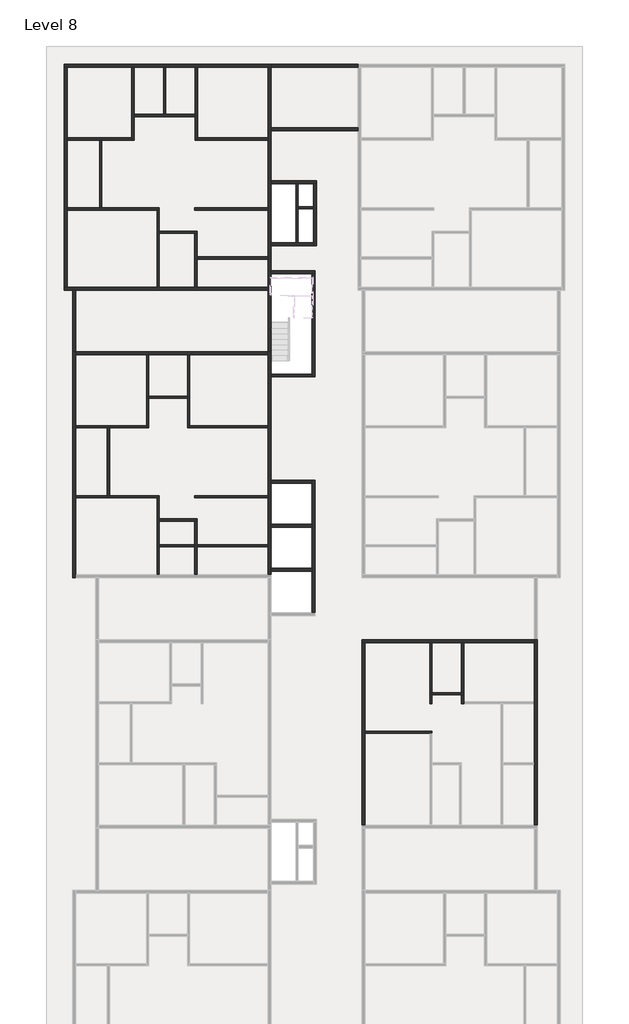
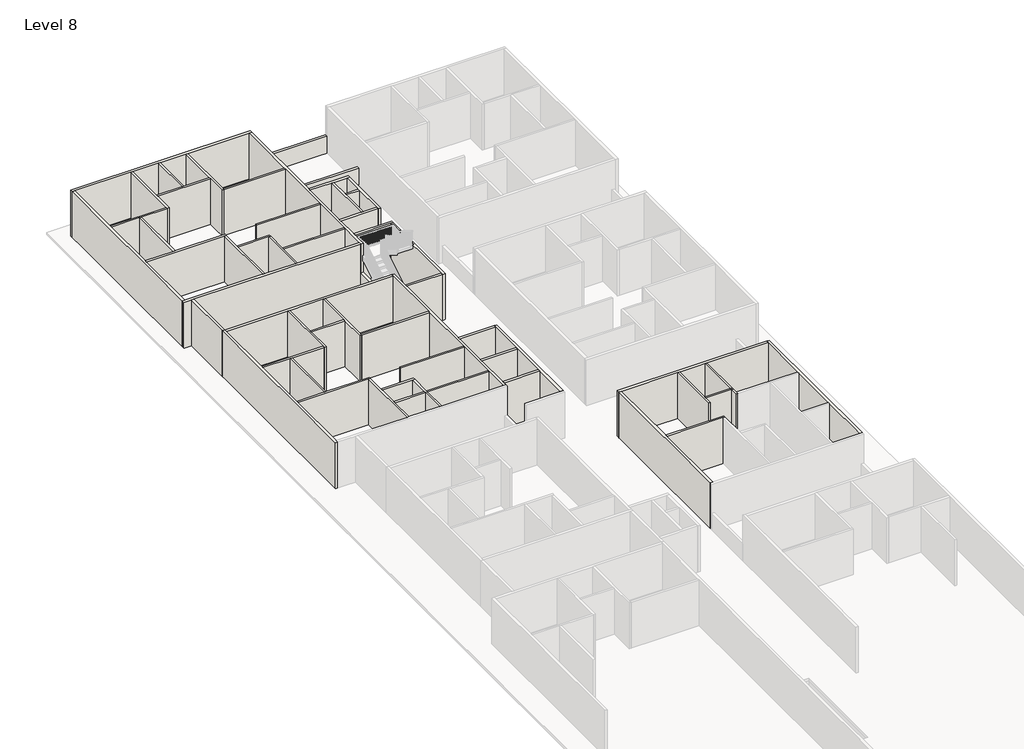
# One storey, part 3 of 8: 57 walls.
"""IFC4 building model written with IfcOpenShell, lengths in millimetres."""

from ifc_helpers import new_model, si_unit, frame, origin, place, context, project, spatial, polyline, outline, extrude, faceted_brep, element, save

model = new_model("IFC4")

# Units and contexts
model_context = context("Model", 3, world=origin())
ifc_project = project(units=[si_unit("LENGTHUNIT", "METRE", prefix="MILLI")], contexts=[model_context])

# Site, building, storey
site = spatial("IfcSite", under=ifc_project)
building = spatial("IfcBuilding", under=site)
storey = spatial("IfcBuildingStorey", under=building, Name="Level 8", Elevation=46570.6172466)

# Walls
placement = place(None, origin())
element("IfcWall", 1, ObjectType="4.5\"", at=placement, inside=storey, context=model_context, shape_type="Brep", body=[
    faceted_brep([(-10818.3415084, 35031.1216096, 46570.6172466), (-10818.3415084, 31373.5216096, 46570.6172466), (-10818.3415084, 31259.2216096, 46570.6172466), (-10818.3415084, 31259.2216096, 49618.6172466), (-10818.3415084, 31373.5216096, 49618.6172466), (-10818.3415084, 35031.1216096, 49618.6172466), (-10704.0415084, 35031.1216096, 46570.6172466), (-10704.0415084, 35031.1216096, 49618.6172466), (-10704.0415084, 32592.7216096, 49618.6172466), (-10704.0415084, 32478.4216096, 49618.6172466), (-10704.0415084, 31259.2216096, 49618.6172466), (-10704.0415084, 31259.2216096, 46570.6172466), (-10704.0415084, 32478.4216096, 46570.6172466), (-10704.0415084, 32592.7216096, 46570.6172466)], [[[0, 1, 2, 3, 4, 5]], [[6, 7, 8, 9, 10, 11, 12, 13]], [[2, 1, 0, 6, 13, 12, 11]], [[0, 5, 7, 6]], [[3, 2, 11, 10]], [[5, 4, 3, 10, 9, 8, 7]]]),
])
element("IfcWall", 2, ObjectType="4.5\"", at=placement, inside=storey, context=model_context, shape_type="Brep", body=[
    faceted_brep([(-10818.3415084, 31373.5216096, 46570.6172466), (-14171.1415084, 31373.5216096, 46570.6172466), (-14171.1415084, 31373.5216096, 49618.6172466), (-10818.3415084, 31373.5216096, 49618.6172466), (-10818.3415084, 31259.2216096, 46570.6172466), (-10818.3415084, 31259.2216096, 49618.6172466), (-12380.4415084, 31259.2216096, 49618.6172466), (-12494.7415084, 31259.2216096, 49618.6172466), (-14171.1415084, 31259.2216096, 49618.6172466), (-14171.1415084, 31259.2216096, 46570.6172466), (-12494.7415084, 31259.2216096, 46570.6172466), (-12380.4415084, 31259.2216096, 46570.6172466)], [[[0, 1, 2, 3]], [[4, 5, 6, 7, 8, 9, 10, 11]], [[1, 0, 4, 11, 10, 9]], [[0, 3, 5, 4]], [[2, 1, 9, 8]], [[3, 2, 8, 7, 6, 5]]]),
])
element("IfcWall", 3, ObjectType="4.5\"", at=placement, inside=storey, context=model_context, shape_type="SweptSolid", body=[
    extrude(outline(polyline([(-12494.7415084, 27754.0216096), (-12494.7415084, 31259.2216096), (-12380.4415084, 31259.2216096), (-12380.4415084, 27754.0216096), (-12494.7415084, 27754.0216096)])), frame((0.0, 0.0, 46570.6172466), z_axis=(0.0, 0.0, 1.0), x_axis=(1.0, 0.0, 0.0)), (0.0, 0.0, 1.0), 3048.0),
])
element("IfcWall", 4, ObjectType="4.5\"", at=placement, inside=storey, context=model_context, shape_type="Brep", body=[
    faceted_brep([(-14171.1415084, 27639.7216096, 46570.6172466), (-9510.2415084, 27639.7216096, 46570.6172466), (-9395.9415084, 27639.7216096, 46570.6172466), (-9395.9415084, 27639.7216096, 49618.6172466), (-9510.2415084, 27639.7216096, 49618.6172466), (-14171.1415084, 27639.7216096, 49618.6172466), (-14171.1415084, 27754.0216096, 46570.6172466), (-14171.1415084, 27754.0216096, 49618.6172466), (-12494.7415084, 27754.0216096, 49618.6172466), (-12380.4415084, 27754.0216096, 49618.6172466), (-9395.9415084, 27754.0216096, 49618.6172466), (-9395.9415084, 27754.0216096, 46570.6172466), (-12380.4415084, 27754.0216096, 46570.6172466), (-12494.7415084, 27754.0216096, 46570.6172466)], [[[0, 1, 2, 3, 4, 5]], [[6, 7, 8, 9, 10, 11, 12, 13]], [[2, 1, 0, 6, 13, 12, 11]], [[0, 5, 7, 6]], [[3, 2, 11, 10]], [[5, 4, 3, 10, 9, 8, 7]]]),
])
element("IfcWall", 5, ObjectType="4.5\"", at=placement, inside=storey, context=model_context, shape_type="Brep", body=[
    faceted_brep([(-9510.2415084, 27639.7216096, 46570.6172466), (-9510.2415084, 23651.9216096, 46570.6172466), (-9510.2415084, 23651.9216096, 49618.6172466), (-9510.2415084, 27639.7216096, 49618.6172466), (-9395.9415084, 27639.7216096, 46570.6172466), (-9395.9415084, 27639.7216096, 49618.6172466), (-9395.9415084, 26547.5216096, 49618.6172466), (-9395.9415084, 26433.2216096, 49618.6172466), (-9395.9415084, 23651.9216096, 49618.6172466), (-9395.9415084, 23651.9216096, 46570.6172466), (-9395.9415084, 26433.2216096, 46570.6172466), (-9395.9415084, 26547.5216096, 46570.6172466)], [[[0, 1, 2, 3]], [[4, 5, 6, 7, 8, 9, 10, 11]], [[1, 0, 4, 11, 10, 9]], [[0, 3, 5, 4]], [[2, 1, 9, 8]], [[3, 2, 8, 7, 6, 5]]]),
])
element("IfcWall", 6, ObjectType="4.5\"", at=placement, inside=storey, context=model_context, shape_type="Brep", body=[
    faceted_brep([(-9395.9415084, 26433.2216096, 46570.6172466), (-7567.1415084, 26433.2216096, 46570.6172466), (-7452.8415084, 26433.2216096, 46570.6172466), (-7452.8415084, 26433.2216096, 49618.6172466), (-7567.1415084, 26433.2216096, 49618.6172466), (-9395.9415084, 26433.2216096, 49618.6172466), (-9395.9415084, 26547.5216096, 46570.6172466), (-9395.9415084, 26547.5216096, 49618.6172466), (-7452.8415084, 26547.5216096, 49618.6172466), (-7452.8415084, 26547.5216096, 46570.6172466)], [[[0, 1, 2, 3, 4, 5]], [[6, 7, 8, 9]], [[2, 1, 0, 6, 9]], [[0, 5, 7, 6]], [[3, 2, 9, 8]], [[5, 4, 3, 8, 7]]]),
])
element("IfcWall", 7, ObjectType="4.5\"", at=placement, inside=storey, context=model_context, shape_type="Brep", body=[
    faceted_brep([(-7567.1415084, 26433.2216096, 46570.6172466), (-7567.1415084, 23651.9216096, 46570.6172466), (-7567.1415084, 23651.9216096, 49618.6172466), (-7567.1415084, 26433.2216096, 49618.6172466), (-7452.8415084, 26433.2216096, 46570.6172466), (-7452.8415084, 26433.2216096, 49618.6172466), (-7452.8415084, 25214.0216096, 49618.6172466), (-7452.8415084, 25099.7216096, 49618.6172466), (-7452.8415084, 23651.9216096, 49618.6172466), (-7452.8415084, 23651.9216096, 46570.6172466), (-7452.8415084, 25099.7216096, 46570.6172466), (-7452.8415084, 25214.0216096, 46570.6172466)], [[[0, 1, 2, 3]], [[4, 5, 6, 7, 8, 9, 10, 11]], [[1, 0, 4, 11, 10, 9]], [[0, 3, 5, 4]], [[2, 1, 9, 8]], [[3, 2, 8, 7, 6, 5]]]),
])
element("IfcWall", 8, ObjectType="4.5\"", at=placement, inside=storey, context=model_context, shape_type="SweptSolid", body=[
    extrude(outline(polyline([(-7452.8415084, 25214.0216096), (-3769.8415084, 25214.0216096), (-3769.8415084, 25099.7216096), (-7452.8415084, 25099.7216096), (-7452.8415084, 25214.0216096)])), frame((0.0, 0.0, 46570.6172466), z_axis=(0.0, 0.0, 1.0), x_axis=(1.0, 0.0, 0.0)), (0.0, 0.0, 1.0), 3048.0),
])
element("IfcWall", 9, ObjectType="4.5\"", at=placement, inside=storey, context=model_context, shape_type="SweptSolid", body=[
    extrude(outline(polyline([(-3769.8415084, 27639.7216096), (-7567.1415084, 27639.7216096), (-7567.1415084, 27754.0216096), (-3769.8415084, 27754.0216096), (-3769.8415084, 27639.7216096)])), frame((0.0, 0.0, 46570.6172466), z_axis=(0.0, 0.0, 1.0), x_axis=(1.0, 0.0, 0.0)), (0.0, 0.0, 1.0), 3048.0),
])
element("IfcWall", 10, ObjectType="4.5\"", at=placement, inside=storey, context=model_context, shape_type="Brep", body=[
    faceted_brep([(-10704.0415084, 32478.4216096, 46570.6172466), (-7541.7415084, 32478.4216096, 46570.6172466), (-7541.7415084, 32478.4216096, 49618.6172466), (-10704.0415084, 32478.4216096, 49618.6172466), (-10704.0415084, 32592.7216096, 46570.6172466), (-10704.0415084, 32592.7216096, 49618.6172466), (-9180.0415084, 32592.7216096, 49618.6172466), (-9065.7415084, 32592.7216096, 49618.6172466), (-7541.7415084, 32592.7216096, 49618.6172466), (-7541.7415084, 32592.7216096, 46570.6172466), (-9065.7415084, 32592.7216096, 46570.6172466), (-9180.0415084, 32592.7216096, 46570.6172466)], [[[0, 1, 2, 3]], [[4, 5, 6, 7, 8, 9, 10, 11]], [[1, 0, 4, 11, 10, 9]], [[0, 3, 5, 4]], [[2, 1, 9, 8]], [[3, 2, 8, 7, 6, 5]]]),
])
element("IfcWall", 11, ObjectType="4.5\"", at=placement, inside=storey, context=model_context, shape_type="SweptSolid", body=[
    extrude(outline(polyline([(-9180.0415084, 32592.7216096), (-9180.0415084, 35031.1216096), (-9065.7415084, 35031.1216096), (-9065.7415084, 32592.7216096), (-9180.0415084, 32592.7216096)])), frame((0.0, 0.0, 46570.6172466), z_axis=(0.0, 0.0, 1.0), x_axis=(1.0, 0.0, 0.0)), (0.0, 0.0, 1.0), 3048.0),
])
element("IfcWall", 12, ObjectType="4.5\"", at=placement, inside=storey, context=model_context, shape_type="Brep", body=[
    faceted_brep([(-7541.7415084, 35031.1216096, 46570.6172466), (-7541.7415084, 32592.7216096, 46570.6172466), (-7541.7415084, 32478.4216096, 46570.6172466), (-7541.7415084, 31259.2216096, 46570.6172466), (-7541.7415084, 31259.2216096, 49618.6172466), (-7541.7415084, 32478.4216096, 49618.6172466), (-7541.7415084, 32592.7216096, 49618.6172466), (-7541.7415084, 35031.1216096, 49618.6172466), (-7427.4415084, 35031.1216096, 46570.6172466), (-7427.4415084, 35031.1216096, 49618.6172466), (-7427.4415084, 31373.5216096, 49618.6172466), (-7427.4415084, 31259.2216096, 49618.6172466), (-7427.4415084, 31259.2216096, 46570.6172466), (-7427.4415084, 31373.5216096, 46570.6172466)], [[[0, 1, 2, 3, 4, 5, 6, 7]], [[8, 9, 10, 11, 12, 13]], [[3, 2, 1, 0, 8, 13, 12]], [[0, 7, 9, 8]], [[4, 3, 12, 11]], [[7, 6, 5, 4, 11, 10, 9]]]),
])
element("IfcWall", 13, ObjectType="4.5\"", at=placement, inside=storey, context=model_context, shape_type="SweptSolid", body=[
    extrude(outline(polyline([(-3769.8415084, 31259.2216096), (-7427.4415084, 31259.2216096), (-7427.4415084, 31373.5216096), (-3769.8415084, 31373.5216096), (-3769.8415084, 31259.2216096)])), frame((0.0, 0.0, 46570.6172466), z_axis=(0.0, 0.0, 1.0), x_axis=(1.0, 0.0, 0.0)), (0.0, 0.0, 1.0), 3048.0),
])
element("IfcWall", 14, ObjectType="4.5\"", at=placement, inside=storey, context=model_context, shape_type="Brep", body=[
    faceted_brep([(-10061.4044854, 20146.7216096, 46570.6172466), (-10061.4044854, 16489.1216096, 46570.6172466), (-10061.4044854, 16374.8216096, 46570.6172466), (-10061.4044854, 16374.8216096, 49618.6172466), (-10061.4044854, 16489.1216096, 49618.6172466), (-10061.4044854, 20146.7216096, 49618.6172466), (-9947.1044854, 20146.7216096, 46570.6172466), (-9947.1044854, 20146.7216096, 49618.6172466), (-9947.1044854, 18013.1216096, 49618.6172466), (-9947.1044854, 17898.8216096, 49618.6172466), (-9947.1044854, 16374.8216096, 49618.6172466), (-9947.1044854, 16374.8216096, 46570.6172466), (-9947.1044854, 17898.8216096, 46570.6172466), (-9947.1044854, 18013.1216096, 46570.6172466)], [[[0, 1, 2, 3, 4, 5]], [[6, 7, 8, 9, 10, 11, 12, 13]], [[2, 1, 0, 6, 13, 12, 11]], [[0, 5, 7, 6]], [[3, 2, 11, 10]], [[5, 4, 3, 10, 9, 8, 7]]]),
])
element("IfcWall", 15, ObjectType="4.5\"", at=placement, inside=storey, context=model_context, shape_type="Brep", body=[
    faceted_brep([(-10061.4044854, 16489.1216096, 46570.6172466), (-13719.0044854, 16489.1216096, 46570.6172466), (-13719.0044854, 16489.1216096, 49618.6172466), (-10061.4044854, 16489.1216096, 49618.6172466), (-10061.4044854, 16374.8216096, 46570.6172466), (-10061.4044854, 16374.8216096, 49618.6172466), (-11980.3915084, 16374.8216096, 49618.6172466), (-12094.6915084, 16374.8216096, 49618.6172466), (-13719.0044854, 16374.8216096, 49618.6172466), (-13719.0044854, 16374.8216096, 46570.6172466), (-12094.6915084, 16374.8216096, 46570.6172466), (-11980.3915084, 16374.8216096, 46570.6172466)], [[[0, 1, 2, 3]], [[4, 5, 6, 7, 8, 9, 10, 11]], [[1, 0, 4, 11, 10, 9]], [[0, 3, 5, 4]], [[2, 1, 9, 8]], [[3, 2, 8, 7, 6, 5]]]),
])
element("IfcWall", 16, ObjectType="4.5\"", at=placement, inside=storey, context=model_context, shape_type="SweptSolid", body=[
    extrude(outline(polyline([(-7940.5044854, 17898.8216096), (-9947.1044854, 17898.8216096), (-9947.1044854, 18013.1216096), (-7940.5044854, 18013.1216096), (-7940.5044854, 17898.8216096)])), frame((0.0, 0.0, 46570.6172466), z_axis=(0.0, 0.0, 1.0), x_axis=(1.0, 0.0, 0.0)), (0.0, 0.0, 1.0), 3048.0),
])
element("IfcWall", 17, ObjectType="4.5\"", at=placement, inside=storey, context=model_context, shape_type="Brep", body=[
    faceted_brep([(-7940.5044854, 20146.7216096, 46570.6172466), (-7940.5044854, 18013.1216096, 46570.6172466), (-7940.5044854, 17898.8216096, 46570.6172466), (-7940.5044854, 16374.8216096, 46570.6172466), (-7940.5044854, 16374.8216096, 49618.6172466), (-7940.5044854, 17898.8216096, 49618.6172466), (-7940.5044854, 18013.1216096, 49618.6172466), (-7940.5044854, 20146.7216096, 49618.6172466), (-7826.2044854, 20146.7216096, 46570.6172466), (-7826.2044854, 20146.7216096, 49618.6172466), (-7826.2044854, 16489.1216096, 49618.6172466), (-7826.2044854, 16374.8216096, 49618.6172466), (-7826.2044854, 16374.8216096, 46570.6172466), (-7826.2044854, 16489.1216096, 46570.6172466)], [[[0, 1, 2, 3, 4, 5, 6, 7]], [[8, 9, 10, 11, 12, 13]], [[3, 2, 1, 0, 8, 13, 12]], [[0, 7, 9, 8]], [[4, 3, 12, 11]], [[7, 6, 5, 4, 11, 10, 9]]]),
])
element("IfcWall", 18, ObjectType="4.5\"", at=placement, inside=storey, context=model_context, shape_type="SweptSolid", body=[
    extrude(outline(polyline([(-3769.8415084, 16374.8216096), (-7826.2044854, 16374.8216096), (-7826.2044854, 16489.1216096), (-3769.8415084, 16489.1216096), (-3769.8415084, 16374.8216096)])), frame((0.0, 0.0, 46570.6172466), z_axis=(0.0, 0.0, 1.0), x_axis=(1.0, 0.0, 0.0)), (0.0, 0.0, 1.0), 3048.0),
])
element("IfcWall", 19, ObjectType="4.5\"", at=placement, inside=storey, context=model_context, shape_type="SweptSolid", body=[
    extrude(outline(polyline([(-12094.6915084, 12869.6216096), (-12094.6915084, 16374.8216096), (-11980.3915084, 16374.8216096), (-11980.3915084, 12869.6216096), (-12094.6915084, 12869.6216096)])), frame((0.0, 0.0, 46570.6172466), z_axis=(0.0, 0.0, 1.0), x_axis=(1.0, 0.0, 0.0)), (0.0, 0.0, 1.0), 3048.0),
])
element("IfcWall", 20, ObjectType="4.5\"", at=placement, inside=storey, context=model_context, shape_type="Brep", body=[
    faceted_brep([(-13719.0044854, 12755.3216096, 46570.6172466), (-9510.2415084, 12755.3216096, 46570.6172466), (-9395.9415084, 12755.3216096, 46570.6172466), (-9395.9415084, 12755.3216096, 49618.6172466), (-9510.2415084, 12755.3216096, 49618.6172466), (-13719.0044854, 12755.3216096, 49618.6172466), (-13719.0044854, 12869.6216096, 46570.6172466), (-13719.0044854, 12869.6216096, 49618.6172466), (-12094.6915084, 12869.6216096, 49618.6172466), (-11980.3915084, 12869.6216096, 49618.6172466), (-9395.9415084, 12869.6216096, 49618.6172466), (-9395.9415084, 12869.6216096, 46570.6172466), (-11980.3915084, 12869.6216096, 46570.6172466), (-12094.6915084, 12869.6216096, 46570.6172466)], [[[0, 1, 2, 3, 4, 5]], [[6, 7, 8, 9, 10, 11, 12, 13]], [[2, 1, 0, 6, 13, 12, 11]], [[0, 5, 7, 6]], [[3, 2, 11, 10]], [[5, 4, 3, 10, 9, 8, 7]]]),
])
element("IfcWall", 21, ObjectType="4.5\"", at=placement, inside=storey, context=model_context, shape_type="Brep", body=[
    faceted_brep([(-9510.2415084, 12755.3216096, 46570.6172466), (-9510.2415084, 8767.5216096, 46570.6172466), (-9510.2415084, 8767.5216096, 49618.6172466), (-9510.2415084, 12755.3216096, 49618.6172466), (-9395.9415084, 12755.3216096, 46570.6172466), (-9395.9415084, 12755.3216096, 49618.6172466), (-9395.9415084, 11663.1216096, 49618.6172466), (-9395.9415084, 11548.8216096, 49618.6172466), (-9395.9415084, 10329.6216096, 49618.6172466), (-9395.9415084, 10215.3216096, 49618.6172466), (-9395.9415084, 8767.5216096, 49618.6172466), (-9395.9415084, 8767.5216096, 46570.6172466), (-9395.9415084, 10215.3216096, 46570.6172466), (-9395.9415084, 10329.6216096, 46570.6172466), (-9395.9415084, 11548.8216096, 46570.6172466), (-9395.9415084, 11663.1216096, 46570.6172466)], [[[0, 1, 2, 3]], [[4, 5, 6, 7, 8, 9, 10, 11, 12, 13, 14, 15]], [[1, 0, 4, 15, 14, 13, 12, 11]], [[0, 3, 5, 4]], [[2, 1, 11, 10]], [[3, 2, 10, 9, 8, 7, 6, 5]]]),
])
element("IfcWall", 22, ObjectType="4.5\"", at=placement, inside=storey, context=model_context, shape_type="SweptSolid", body=[
    extrude(outline(polyline([(-7567.1415084, 10215.3216096), (-9395.9415084, 10215.3216096), (-9395.9415084, 10329.6216096), (-7567.1415084, 10329.6216096), (-7567.1415084, 10215.3216096)])), frame((0.0, 0.0, 46570.6172466), z_axis=(0.0, 0.0, 1.0), x_axis=(1.0, 0.0, 0.0)), (0.0, 0.0, 1.0), 3048.0),
])
element("IfcWall", 23, ObjectType="4.5\"", at=placement, inside=storey, context=model_context, shape_type="Brep", body=[
    faceted_brep([(-9395.9415084, 11548.8216096, 46570.6172466), (-7567.1415084, 11548.8216096, 46570.6172466), (-7452.8415084, 11548.8216096, 46570.6172466), (-7452.8415084, 11548.8216096, 49618.6172466), (-7567.1415084, 11548.8216096, 49618.6172466), (-9395.9415084, 11548.8216096, 49618.6172466), (-9395.9415084, 11663.1216096, 46570.6172466), (-9395.9415084, 11663.1216096, 49618.6172466), (-7452.8415084, 11663.1216096, 49618.6172466), (-7452.8415084, 11663.1216096, 46570.6172466)], [[[0, 1, 2, 3, 4, 5]], [[6, 7, 8, 9]], [[2, 1, 0, 6, 9]], [[0, 5, 7, 6]], [[3, 2, 9, 8]], [[5, 4, 3, 8, 7]]]),
])
element("IfcWall", 24, ObjectType="4.5\"", at=placement, inside=storey, context=model_context, shape_type="Brep", body=[
    faceted_brep([(-7567.1415084, 11548.8216096, 46570.6172466), (-7567.1415084, 10329.6216096, 46570.6172466), (-7567.1415084, 10215.3216096, 46570.6172466), (-7567.1415084, 8767.5216096, 46570.6172466), (-7567.1415084, 8767.5216096, 49618.6172466), (-7567.1415084, 10215.3216096, 49618.6172466), (-7567.1415084, 10329.6216096, 49618.6172466), (-7567.1415084, 11548.8216096, 49618.6172466), (-7452.8415084, 11548.8216096, 46570.6172466), (-7452.8415084, 11548.8216096, 49618.6172466), (-7452.8415084, 10329.6216096, 49618.6172466), (-7452.8415084, 10215.3216096, 49618.6172466), (-7452.8415084, 8767.5216096, 49618.6172466), (-7452.8415084, 8767.5216096, 46570.6172466), (-7452.8415084, 10215.3216096, 46570.6172466), (-7452.8415084, 10329.6216096, 46570.6172466)], [[[0, 1, 2, 3, 4, 5, 6, 7]], [[8, 9, 10, 11, 12, 13, 14, 15]], [[3, 2, 1, 0, 8, 15, 14, 13]], [[0, 7, 9, 8]], [[4, 3, 13, 12]], [[7, 6, 5, 4, 12, 11, 10, 9]]]),
])
element("IfcWall", 25, ObjectType="4.5\"", at=placement, inside=storey, context=model_context, shape_type="SweptSolid", body=[
    extrude(outline(polyline([(-3769.8415084, 10215.3216096), (-7452.8415084, 10215.3216096), (-7452.8415084, 10329.6216096), (-3769.8415084, 10329.6216096), (-3769.8415084, 10215.3216096)])), frame((0.0, 0.0, 46570.6172466), z_axis=(0.0, 0.0, 1.0), x_axis=(1.0, 0.0, 0.0)), (0.0, 0.0, 1.0), 3048.0),
])
element("IfcWall", 26, ObjectType="4.5\"", at=placement, inside=storey, context=model_context, shape_type="SweptSolid", body=[
    extrude(outline(polyline([(-3769.8415084, 12755.3216096), (-7567.1415084, 12755.3216096), (-7567.1415084, 12869.6216096), (-3769.8415084, 12869.6216096), (-3769.8415084, 12755.3216096)])), frame((0.0, 0.0, 46570.6172466), z_axis=(0.0, 0.0, 1.0), x_axis=(1.0, 0.0, 0.0)), (0.0, 0.0, 1.0), 3048.0),
])
element("IfcWall", 27, ObjectType="4.5\"", at=placement, inside=storey, context=model_context, shape_type="Brep", body=[
    faceted_brep([(1259.3584916, 572.7745083, 46570.6172466), (4610.8714687, 572.7745083, 46570.6172466), (4725.1714687, 572.7745083, 46570.6172466), (4725.1714687, 572.7745083, 49618.6172466), (4610.8714687, 572.7745083, 49618.6172466), (1259.3584916, 572.7745083, 49618.6172466), (1259.3584916, 687.0745083, 46570.6172466), (1259.3584916, 687.0745083, 49618.6172466), (4725.1714687, 687.0745083, 49618.6172466), (4725.1714687, 687.0745083, 46570.6172466)], [[[0, 1, 2, 3, 4, 5]], [[6, 7, 8, 9]], [[2, 1, 0, 6, 9]], [[0, 5, 7, 6]], [[3, 2, 9, 8]], [[5, 4, 3, 8, 7]]]),
])
element("IfcWall", 28, ObjectType="4.5\"", at=placement, inside=storey, context=model_context, shape_type="Brep", body=[
    faceted_brep([(4610.8714687, 5262.3216096, 46570.6172466), (4610.8714687, 2100.0216096, 46570.6172466), (4610.8714687, 2100.0216096, 49618.6172466), (4610.8714687, 5262.3216096, 49618.6172466), (4725.1714687, 5262.3216096, 46570.6172466), (4725.1714687, 5262.3216096, 49618.6172466), (4725.1714687, 2671.5216096, 49618.6172466), (4725.1714687, 2557.2216096, 49618.6172466), (4725.1714687, 2100.0216096, 49618.6172466), (4725.1714687, 2100.0216096, 46570.6172466), (4725.1714687, 2557.2216096, 46570.6172466), (4725.1714687, 2671.5216096, 46570.6172466)], [[[0, 1, 2, 3]], [[4, 5, 6, 7, 8, 9, 10, 11]], [[1, 0, 4, 11, 10, 9]], [[2, 1, 9, 8]], [[0, 3, 5, 4]], [[3, 2, 8, 7, 6, 5]]]),
])
element("IfcWall", 29, ObjectType="4.5\"", at=placement, inside=storey, context=model_context, shape_type="Brep", body=[
    faceted_brep([(4725.1714687, 2557.2216096, 46570.6172466), (6249.1714687, 2557.2216096, 46570.6172466), (6363.4714687, 2557.2216096, 46570.6172466), (6363.4714687, 2557.2216096, 49618.6172466), (6249.1714687, 2557.2216096, 49618.6172466), (4725.1714687, 2557.2216096, 49618.6172466), (4725.1714687, 2671.5216096, 46570.6172466), (4725.1714687, 2671.5216096, 49618.6172466), (6249.1714687, 2671.5216096, 49618.6172466), (6363.4714687, 2671.5216096, 49618.6172466), (6363.4714687, 2671.5216096, 46570.6172466), (6249.1714687, 2671.5216096, 46570.6172466)], [[[0, 1, 2, 3, 4, 5]], [[6, 7, 8, 9, 10, 11]], [[2, 1, 0, 6, 11, 10]], [[0, 5, 7, 6]], [[3, 2, 10, 9]], [[5, 4, 3, 9, 8, 7]]]),
])
element("IfcWall", 30, ObjectType="4.5\"", at=placement, inside=storey, context=model_context, shape_type="SweptSolid", body=[
    extrude(outline(polyline([(6363.4714687, 5262.3216096), (6363.4714687, 2671.5216096), (6249.1714687, 2671.5216096), (6249.1714687, 5262.3216096), (6363.4714687, 5262.3216096)])), frame((0.0, 0.0, 46570.6172466), z_axis=(0.0, 0.0, 1.0), x_axis=(1.0, 0.0, 0.0)), (0.0, 0.0, 1.0), 3048.0),
])
element("IfcWall", 31, ObjectType="4.5\"", at=placement, inside=storey, context=model_context, shape_type="Brep", body=[
    faceted_brep([(6249.1714687, 2557.2216096, 46570.6172466), (6249.1714687, 2100.0216096, 46570.6172466), (6249.1714687, 2100.0216096, 49618.6172466), (6249.1714687, 2557.2216096, 49618.6172466), (6363.4714687, 2557.2216096, 46570.6172466), (6363.4714687, 2557.2216096, 49618.6172466), (6363.4714687, 2214.3216096, 49618.6172466), (6363.4714687, 2100.0216096, 49618.6172466), (6363.4714687, 2100.0216096, 46570.6172466), (6363.4714687, 2214.3216096, 46570.6172466)], [[[0, 1, 2, 3]], [[4, 5, 6, 7, 8, 9]], [[1, 0, 4, 9, 8]], [[0, 3, 5, 4]], [[2, 1, 8, 7]], [[3, 2, 7, 6, 5]]]),
])
element("IfcWall", 32, ObjectType="4.5\"", at=placement, inside=storey, context=model_context, shape_type="Brep", body=[
    faceted_brep([(-2321.9738684, 29000.0900967, 46570.6172466), (-2321.9738684, 25952.0900967, 46570.6172466), (-2321.9738684, 25952.0900967, 49618.6172466), (-2321.9738684, 29000.0900967, 49618.6172466), (-2207.6738684, 29000.0900967, 46570.6172466), (-2207.6738684, 29000.0900967, 49618.6172466), (-2207.6738684, 27820.8172885, 49618.6172466), (-2207.6738684, 27706.5172885, 49618.6172466), (-2207.6738684, 25952.0900967, 49618.6172466), (-2207.6738684, 25952.0900967, 46570.6172466), (-2207.6738684, 27706.5172885, 46570.6172466), (-2207.6738684, 27820.8172885, 46570.6172466)], [[[0, 1, 2, 3]], [[4, 5, 6, 7, 8, 9, 10, 11]], [[1, 0, 4, 11, 10, 9]], [[3, 2, 8, 7, 6, 5]], [[0, 3, 5, 4]], [[2, 1, 9, 8]]]),
])
element("IfcWall", 33, ObjectType="4.5\"", at=placement, inside=storey, context=model_context, shape_type="SweptSolid", body=[
    extrude(outline(polyline([(-2207.6738684, 27820.8172885), (-1407.6415084, 27820.8172885), (-1407.6415084, 27706.5172885), (-2207.6738684, 27706.5172885), (-2207.6738684, 27820.8172885)])), frame((0.0, 0.0, 46570.6172466), z_axis=(0.0, 0.0, 1.0), x_axis=(1.0, 0.0, 0.0)), (0.0, 0.0, 1.0), 3048.0),
])
element("IfcWall", 34, ObjectType="6\"", at=placement, inside=storey, context=model_context, shape_type="Brep", body=[
    faceted_brep([(-14323.5415084, 35031.1216096, 46570.6172466), (-14171.1415084, 35031.1216096, 46570.6172466), (-10818.3415084, 35031.1216096, 46570.6172466), (-10704.0415084, 35031.1216096, 46570.6172466), (-9180.0415084, 35031.1216096, 46570.6172466), (-9065.7415084, 35031.1216096, 46570.6172466), (-7541.7415084, 35031.1216096, 46570.6172466), (-7427.4415084, 35031.1216096, 46570.6172466), (-3769.8415084, 35031.1216096, 46570.6172466), (-3617.4415084, 35031.1216096, 46570.6172466), (-3617.4415084, 35031.1216096, 49618.6172466), (-3769.8415084, 35031.1216096, 49618.6172466), (-7427.4415084, 35031.1216096, 49618.6172466), (-7541.7415084, 35031.1216096, 49618.6172466), (-9065.7415084, 35031.1216096, 49618.6172466), (-9180.0415084, 35031.1216096, 49618.6172466), (-10704.0415084, 35031.1216096, 49618.6172466), (-10818.3415084, 35031.1216096, 49618.6172466), (-14171.1415084, 35031.1216096, 49618.6172466), (-14323.5415084, 35031.1216096, 49618.6172466), (-14323.5415084, 35183.5216096, 46570.6172466), (-14323.5415084, 35183.5216096, 49618.6172466), (-3617.4415084, 35183.5216096, 49618.6172466), (-3617.4415084, 35183.5216096, 46570.6172466)], [[[0, 1, 2, 3, 4, 5, 6, 7, 8, 9, 10, 11, 12, 13, 14, 15, 16, 17, 18, 19]], [[20, 21, 22, 23]], [[9, 8, 7, 6, 5, 4, 3, 2, 1, 0, 20, 23]], [[0, 19, 21, 20]], [[9, 23, 22, 10]], [[19, 18, 17, 16, 15, 14, 13, 12, 11, 10, 22, 21]]]),
])
element("IfcWall", 35, ObjectType="6\"", at=placement, inside=storey, context=model_context, shape_type="Brep", body=[
    faceted_brep([(-3769.8415084, 35031.1216096, 49618.6172466), (-3769.8415084, 35031.1216096, 46570.6172466), (-3769.8415084, 31373.5216096, 46570.6172466), (-3769.8415084, 31259.2216096, 46570.6172466), (-3769.8415084, 27754.0216096, 46570.6172466), (-3769.8415084, 27639.7216096, 46570.6172466), (-3769.8415084, 25214.0216096, 46570.6172466), (-3769.8415084, 25099.7216096, 46570.6172466), (-3769.8415084, 23651.9216096, 46570.6172466), (-3769.8415084, 23499.5216096, 46570.6172466), (-3769.8415084, 23499.5216096, 49618.6172466), (-3769.8415084, 23651.9216096, 49618.6172466), (-3769.8415084, 25099.7216096, 49618.6172466), (-3769.8415084, 25214.0216096, 49618.6172466), (-3769.8415084, 27639.7216096, 49618.6172466), (-3769.8415084, 27754.0216096, 49618.6172466), (-3769.8415084, 31259.2216096, 49618.6172466), (-3769.8415084, 31373.5216096, 49618.6172466), (-3617.4415084, 35031.1216096, 46570.6172466), (-3617.4415084, 35031.1216096, 49618.6172466), (-3617.4415084, 29152.4900967, 49618.6172466), (-3617.4415084, 29000.0900967, 49618.6172466), (-3617.4415084, 25952.0900967, 49618.6172466), (-3617.4415084, 25799.6900967, 49618.6172466), (-3617.4415084, 24490.1216096, 49618.6172466), (-3617.4415084, 24337.7216096, 49618.6172466), (-3617.4415084, 23499.5216096, 49618.6172466), (-3617.4415084, 23499.5216096, 46570.6172466), (-3617.4415084, 24337.7216096, 46570.6172466), (-3617.4415084, 24490.1216096, 46570.6172466), (-3617.4415084, 25799.6900967, 46570.6172466), (-3617.4415084, 25952.0900967, 46570.6172466), (-3617.4415084, 29000.0900967, 46570.6172466), (-3617.4415084, 29152.4900967, 46570.6172466), (-3617.4415084, 31744.9197155, 46570.6172466), (-3617.4415084, 31897.3197155, 46570.6172466)], [[[0, 1, 2, 3, 4, 5, 6, 7, 8, 9, 10, 11, 12, 13, 14, 15, 16, 17]], [[18, 19, 20, 21, 22, 23, 24, 25, 26, 27, 28, 29, 30, 31, 32, 33, 34, 35]], [[9, 8, 7, 6, 5, 4, 3, 2, 1, 18, 35, 34, 33, 32, 31, 30, 29, 28, 27]], [[0, 19, 18, 1]], [[9, 27, 26, 10]], [[0, 17, 16, 15, 14, 13, 12, 11, 10, 26, 25, 24, 23, 22, 21, 20, 19]]]),
])
element("IfcWall", 36, ObjectType="6\"", at=placement, inside=storey, context=model_context, shape_type="Brep", body=[
    faceted_brep([(-3769.8415084, 23651.9216096, 49618.6172466), (-3769.8415084, 23651.9216096, 46570.6172466), (-7452.8415084, 23651.9216096, 46570.6172466), (-7567.1415084, 23651.9216096, 46570.6172466), (-9395.9415084, 23651.9216096, 46570.6172466), (-9510.2415084, 23651.9216096, 46570.6172466), (-14171.1415084, 23651.9216096, 46570.6172466), (-14323.5415084, 23651.9216096, 46570.6172466), (-14323.5415084, 23651.9216096, 49618.6172466), (-14171.1415084, 23651.9216096, 49618.6172466), (-9510.2415084, 23651.9216096, 49618.6172466), (-9395.9415084, 23651.9216096, 49618.6172466), (-7567.1415084, 23651.9216096, 49618.6172466), (-7452.8415084, 23651.9216096, 49618.6172466), (-3769.8415084, 23499.5216096, 46570.6172466), (-3769.8415084, 23499.5216096, 49618.6172466), (-13719.0044854, 23499.5216096, 49618.6172466), (-13871.4044854, 23499.5216096, 49618.6172466), (-14323.5415084, 23499.5216096, 49618.6172466), (-14323.5415084, 23499.5216096, 46570.6172466), (-13871.4044854, 23499.5216096, 46570.6172466), (-13719.0044854, 23499.5216096, 46570.6172466)], [[[0, 1, 2, 3, 4, 5, 6, 7, 8, 9, 10, 11, 12, 13]], [[14, 15, 16, 17, 18, 19, 20, 21]], [[7, 6, 5, 4, 3, 2, 1, 14, 21, 20, 19]], [[8, 7, 19, 18]], [[0, 15, 14, 1]], [[0, 13, 12, 11, 10, 9, 8, 18, 17, 16, 15]]]),
])
element("IfcWall", 37, ObjectType="6\"", at=placement, inside=storey, context=model_context, shape_type="Brep", body=[
    faceted_brep([(-14171.1415084, 23651.9216096, 46570.6172466), (-14171.1415084, 27639.7216096, 46570.6172466), (-14171.1415084, 27754.0216096, 46570.6172466), (-14171.1415084, 31259.2216096, 46570.6172466), (-14171.1415084, 31373.5216096, 46570.6172466), (-14171.1415084, 35031.1216096, 46570.6172466), (-14171.1415084, 35031.1216096, 49618.6172466), (-14171.1415084, 31373.5216096, 49618.6172466), (-14171.1415084, 31259.2216096, 49618.6172466), (-14171.1415084, 27754.0216096, 49618.6172466), (-14171.1415084, 27639.7216096, 49618.6172466), (-14171.1415084, 23651.9216096, 49618.6172466), (-14323.5415084, 23651.9216096, 46570.6172466), (-14323.5415084, 23651.9216096, 49618.6172466), (-14323.5415084, 35031.1216096, 49618.6172466), (-14323.5415084, 35031.1216096, 46570.6172466)], [[[0, 1, 2, 3, 4, 5, 6, 7, 8, 9, 10, 11]], [[12, 13, 14, 15]], [[5, 4, 3, 2, 1, 0, 12, 15]], [[6, 5, 15, 14]], [[0, 11, 13, 12]], [[11, 10, 9, 8, 7, 6, 14, 13]]]),
])
element("IfcWall", 38, ObjectType="6\"", at=placement, inside=storey, context=model_context, shape_type="Brep", body=[
    faceted_brep([(-13871.4044854, 20299.1216096, 46570.6172466), (-13871.4044854, 8615.1216096, 46570.6172466), (-13871.4044854, 8615.1216096, 49618.6172466), (-13871.4044854, 20299.1216096, 49618.6172466), (-13719.0044854, 20299.1216096, 46570.6172466), (-13719.0044854, 20299.1216096, 49618.6172466), (-13719.0044854, 20146.7216096, 49618.6172466), (-13719.0044854, 16489.1216096, 49618.6172466), (-13719.0044854, 16374.8216096, 49618.6172466), (-13719.0044854, 12869.6216096, 49618.6172466), (-13719.0044854, 12755.3216096, 49618.6172466), (-13719.0044854, 8767.5216096, 49618.6172466), (-13719.0044854, 8615.1216096, 49618.6172466), (-13719.0044854, 8615.1216096, 46570.6172466), (-13719.0044854, 8767.5216096, 46570.6172466), (-13719.0044854, 12755.3216096, 46570.6172466), (-13719.0044854, 12869.6216096, 46570.6172466), (-13719.0044854, 16374.8216096, 46570.6172466), (-13719.0044854, 16489.1216096, 46570.6172466), (-13719.0044854, 20146.7216096, 46570.6172466)], [[[0, 1, 2, 3]], [[4, 5, 6, 7, 8, 9, 10, 11, 12, 13, 14, 15, 16, 17, 18, 19]], [[1, 0, 4, 19, 18, 17, 16, 15, 14, 13]], [[2, 1, 13, 12]], [[0, 3, 5, 4]], [[3, 2, 12, 11, 10, 9, 8, 7, 6, 5]]]),
])
element("IfcWall", 39, ObjectType="6\"", at=placement, inside=storey, context=model_context, shape_type="Brep", body=[
    faceted_brep([(-3617.4415084, 8767.5216096, 49618.6172466), (-3617.4415084, 8767.5216096, 46570.6172466), (-3617.4415084, 8945.2303368, 46570.6172466), (-3617.4415084, 9097.6303368, 46570.6172466), (-3617.4415084, 11231.2303368, 46570.6172466), (-3617.4415084, 11383.6303368, 46570.6172466), (-3617.4415084, 13517.2303368, 46570.6172466), (-3617.4415084, 13669.6303368, 46570.6172466), (-3617.4415084, 19003.7216096, 46570.6172466), (-3617.4415084, 19156.1216096, 46570.6172466), (-3617.4415084, 20299.1216096, 46570.6172466), (-3617.4415084, 20299.1216096, 49618.6172466), (-3617.4415084, 19156.1216096, 49618.6172466), (-3617.4415084, 19003.7216096, 49618.6172466), (-3617.4415084, 13669.6303368, 49618.6172466), (-3617.4415084, 13517.2303368, 49618.6172466), (-3617.4415084, 11383.6303368, 49618.6172466), (-3617.4415084, 11231.2303368, 49618.6172466), (-3617.4415084, 9097.6303368, 49618.6172466), (-3617.4415084, 8945.2303368, 49618.6172466), (-3769.8415084, 8767.5216096, 46570.6172466), (-3769.8415084, 8767.5216096, 49618.6172466), (-3769.8415084, 10215.3216096, 49618.6172466), (-3769.8415084, 10329.6216096, 49618.6172466), (-3769.8415084, 12755.3216096, 49618.6172466), (-3769.8415084, 12869.6216096, 49618.6172466), (-3769.8415084, 16374.8216096, 49618.6172466), (-3769.8415084, 16489.1216096, 49618.6172466), (-3769.8415084, 20146.7216096, 49618.6172466), (-3769.8415084, 20299.1216096, 49618.6172466), (-3769.8415084, 20299.1216096, 46570.6172466), (-3769.8415084, 20146.7216096, 46570.6172466), (-3769.8415084, 16489.1216096, 46570.6172466), (-3769.8415084, 16374.8216096, 46570.6172466), (-3769.8415084, 12869.6216096, 46570.6172466), (-3769.8415084, 12755.3216096, 46570.6172466), (-3769.8415084, 10329.6216096, 46570.6172466), (-3769.8415084, 10215.3216096, 46570.6172466)], [[[0, 1, 2, 3, 4, 5, 6, 7, 8, 9, 10, 11, 12, 13, 14, 15, 16, 17, 18, 19]], [[20, 21, 22, 23, 24, 25, 26, 27, 28, 29, 30, 31, 32, 33, 34, 35, 36, 37]], [[10, 9, 8, 7, 6, 5, 4, 3, 2, 1, 20, 37, 36, 35, 34, 33, 32, 31, 30]], [[10, 30, 29, 11]], [[0, 21, 20, 1]], [[0, 19, 18, 17, 16, 15, 14, 13, 12, 11, 29, 28, 27, 26, 25, 24, 23, 22, 21]]]),
])
element("IfcWall", 40, ObjectType="6\"", at=placement, inside=storey, context=model_context, shape_type="Brep", body=[
    faceted_brep([(-3769.8415084, 20299.1216096, 49618.6172466), (-3769.8415084, 20299.1216096, 46570.6172466), (-13719.0044854, 20299.1216096, 46570.6172466), (-13719.0044854, 20299.1216096, 49618.6172466), (-3769.8415084, 20146.7216096, 46570.6172466), (-3769.8415084, 20146.7216096, 49618.6172466), (-7826.2044854, 20146.7216096, 49618.6172466), (-7940.5044854, 20146.7216096, 49618.6172466), (-9947.1044854, 20146.7216096, 49618.6172466), (-10061.4044854, 20146.7216096, 49618.6172466), (-13719.0044854, 20146.7216096, 49618.6172466), (-13719.0044854, 20146.7216096, 46570.6172466), (-10061.4044854, 20146.7216096, 46570.6172466), (-9947.1044854, 20146.7216096, 46570.6172466), (-7940.5044854, 20146.7216096, 46570.6172466), (-7826.2044854, 20146.7216096, 46570.6172466)], [[[0, 1, 2, 3]], [[4, 5, 6, 7, 8, 9, 10, 11, 12, 13, 14, 15]], [[2, 1, 4, 15, 14, 13, 12, 11]], [[3, 2, 11, 10]], [[0, 5, 4, 1]], [[0, 3, 10, 9, 8, 7, 6, 5]]]),
])
element("IfcWall", 41, ObjectType="6\"", at=placement, inside=storey, context=model_context, shape_type="Brep", body=[
    faceted_brep([(10173.4714687, -4185.9344126, 49618.6172466), (10173.4714687, -4185.9344126, 46570.6172466), (10173.4714687, 5414.7216096, 46570.6172466), (10173.4714687, 5414.7216096, 49618.6172466), (10021.0714687, -4185.9344126, 46570.6172466), (10021.0714687, -4185.9344126, 49618.6172466), (10021.0714687, -1061.7344126, 49618.6172466), (10021.0714687, -947.4344126, 49618.6172466), (10021.0714687, 2100.0216096, 49618.6172466), (10021.0714687, 2214.3216096, 49618.6172466), (10021.0714687, 5262.3216096, 49618.6172466), (10021.0714687, 5414.7216096, 49618.6172466), (10021.0714687, 5414.7216096, 46570.6172466), (10021.0714687, 5262.3216096, 46570.6172466), (10021.0714687, 2214.3216096, 46570.6172466), (10021.0714687, 2100.0216096, 46570.6172466), (10021.0714687, -947.4344126, 46570.6172466), (10021.0714687, -1061.7344126, 46570.6172466)], [[[0, 1, 2, 3]], [[4, 5, 6, 7, 8, 9, 10, 11, 12, 13, 14, 15, 16, 17]], [[2, 1, 4, 17, 16, 15, 14, 13, 12]], [[2, 12, 11, 3]], [[0, 5, 4, 1]], [[0, 3, 11, 10, 9, 8, 7, 6, 5]]]),
])
element("IfcWall", 42, ObjectType="6\"", at=placement, inside=storey, context=model_context, shape_type="Brep", body=[
    faceted_brep([(10021.0714687, 5414.7216096, 49618.6172466), (10021.0714687, 5414.7216096, 46570.6172466), (1106.9584916, 5414.7216096, 46570.6172466), (1106.9584916, 5414.7216096, 49618.6172466), (10021.0714687, 5262.3216096, 46570.6172466), (10021.0714687, 5262.3216096, 49618.6172466), (6363.4714687, 5262.3216096, 49618.6172466), (6249.1714687, 5262.3216096, 49618.6172466), (4725.1714687, 5262.3216096, 49618.6172466), (4610.8714687, 5262.3216096, 49618.6172466), (1259.3584916, 5262.3216096, 49618.6172466), (1106.9584916, 5262.3216096, 49618.6172466), (1106.9584916, 5262.3216096, 46570.6172466), (1259.3584916, 5262.3216096, 46570.6172466), (4610.8714687, 5262.3216096, 46570.6172466), (4725.1714687, 5262.3216096, 46570.6172466), (6249.1714687, 5262.3216096, 46570.6172466), (6363.4714687, 5262.3216096, 46570.6172466)], [[[0, 1, 2, 3]], [[4, 5, 6, 7, 8, 9, 10, 11, 12, 13, 14, 15, 16, 17]], [[2, 1, 4, 17, 16, 15, 14, 13, 12]], [[3, 2, 12, 11]], [[0, 5, 4, 1]], [[0, 3, 11, 10, 9, 8, 7, 6, 5]]]),
])
element("IfcWall", 43, ObjectType="6\"", at=placement, inside=storey, context=model_context, shape_type="Brep", body=[
    faceted_brep([(1106.9584916, 5262.3216096, 46570.6172466), (1106.9584916, -4185.9344126, 46570.6172466), (1106.9584916, -4185.9344126, 49618.6172466), (1106.9584916, 5262.3216096, 49618.6172466), (1259.3584916, 5262.3216096, 46570.6172466), (1259.3584916, 5262.3216096, 49618.6172466), (1259.3584916, 687.0745083, 49618.6172466), (1259.3584916, 572.7745083, 49618.6172466), (1259.3584916, -4185.9344126, 49618.6172466), (1259.3584916, -4185.9344126, 46570.6172466), (1259.3584916, 572.7745083, 46570.6172466), (1259.3584916, 687.0745083, 46570.6172466)], [[[0, 1, 2, 3]], [[4, 5, 6, 7, 8, 9, 10, 11]], [[1, 0, 4, 11, 10, 9]], [[0, 3, 5, 4]], [[1, 9, 8, 2]], [[3, 2, 8, 7, 6, 5]]]),
])
element("IfcWall", 44, ObjectType="6\"", at=placement, inside=storey, context=model_context, shape_type="Brep", body=[
    faceted_brep([(-1331.4415084, 6811.6303368, 46570.6172466), (-1331.4415084, 13669.6303368, 46570.6172466), (-1331.4415084, 13669.6303368, 49618.6172466), (-1331.4415084, 6811.6303368, 49618.6172466), (-1483.8415084, 6811.6303368, 46570.6172466), (-1483.8415084, 6811.6303368, 49618.6172466), (-1483.8415084, 8945.2303368, 49618.6172466), (-1483.8415084, 9097.6303368, 49618.6172466), (-1483.8415084, 11231.2303368, 49618.6172466), (-1483.8415084, 11383.6303368, 49618.6172466), (-1483.8415084, 13517.2303368, 49618.6172466), (-1483.8415084, 13669.6303368, 49618.6172466), (-1483.8415084, 13669.6303368, 46570.6172466), (-1483.8415084, 13517.2303368, 46570.6172466), (-1483.8415084, 11383.6303368, 46570.6172466), (-1483.8415084, 11231.2303368, 46570.6172466), (-1483.8415084, 9097.6303368, 46570.6172466), (-1483.8415084, 8945.2303368, 46570.6172466)], [[[0, 1, 2, 3]], [[4, 5, 6, 7, 8, 9, 10, 11, 12, 13, 14, 15, 16, 17]], [[1, 0, 4, 17, 16, 15, 14, 13, 12]], [[3, 2, 11, 10, 9, 8, 7, 6, 5]], [[0, 3, 5, 4]], [[2, 1, 12, 11]]]),
])
element("IfcWall", 45, ObjectType="6\"", at=placement, inside=storey, context=model_context, shape_type="SweptSolid", body=[
    extrude(outline(polyline([(-3617.4415084, 13669.6303368), (-1483.8415084, 13669.6303368), (-1483.8415084, 13517.2303368), (-3617.4415084, 13517.2303368), (-3617.4415084, 13669.6303368)])), frame((0.0, 0.0, 46570.6172466), z_axis=(0.0, 0.0, 1.0), x_axis=(1.0, 0.0, 0.0)), (0.0, 0.0, 1.0), 3048.0),
])
element("IfcWall", 46, ObjectType="6\"", at=placement, inside=storey, context=model_context, shape_type="SweptSolid", body=[
    extrude(outline(polyline([(-1483.8415084, 8945.2303368), (-3617.4415084, 8945.2303368), (-3617.4415084, 9097.6303368), (-1483.8415084, 9097.6303368), (-1483.8415084, 8945.2303368)])), frame((0.0, 0.0, 46570.6172466), z_axis=(0.0, 0.0, 1.0), x_axis=(1.0, 0.0, 0.0)), (0.0, 0.0, 1.0), 3048.0),
])
element("IfcWall", 47, ObjectType="6\"", at=placement, inside=storey, context=model_context, shape_type="SweptSolid", body=[
    extrude(outline(polyline([(-3617.4415084, 11383.6303368), (-1483.8415084, 11383.6303368), (-1483.8415084, 11231.2303368), (-3617.4415084, 11231.2303368), (-3617.4415084, 11383.6303368)])), frame((0.0, 0.0, 46570.6172466), z_axis=(0.0, 0.0, 1.0), x_axis=(1.0, 0.0, 0.0)), (0.0, 0.0, 1.0), 3048.0),
])
element("IfcWall", 48, ObjectType="6\"", at=placement, inside=storey, context=model_context, shape_type="Brep", body=[
    faceted_brep([(-3617.4415084, 29000.0900967, 46570.6172466), (-2321.9738684, 29000.0900967, 46570.6172466), (-2207.6738684, 29000.0900967, 46570.6172466), (-1407.6415084, 29000.0900967, 46570.6172466), (-1255.2415084, 29000.0900967, 46570.6172466), (-1255.2415084, 29000.0900967, 49618.6172466), (-1407.6415084, 29000.0900967, 49618.6172466), (-2207.6738684, 29000.0900967, 49618.6172466), (-2321.9738684, 29000.0900967, 49618.6172466), (-3617.4415084, 29000.0900967, 49618.6172466), (-3617.4415084, 29152.4900967, 46570.6172466), (-3617.4415084, 29152.4900967, 49618.6172466), (-1255.2415084, 29152.4900967, 49618.6172466), (-1255.2415084, 29152.4900967, 46570.6172466)], [[[0, 1, 2, 3, 4, 5, 6, 7, 8, 9]], [[10, 11, 12, 13]], [[4, 3, 2, 1, 0, 10, 13]], [[9, 8, 7, 6, 5, 12, 11]], [[0, 9, 11, 10]], [[5, 4, 13, 12]]]),
])
element("IfcWall", 49, ObjectType="6\"", at=placement, inside=storey, context=model_context, shape_type="Brep", body=[
    faceted_brep([(-1407.6415084, 29000.0900967, 46570.6172466), (-1407.6415084, 27820.8172885, 46570.6172466), (-1407.6415084, 27706.5172885, 46570.6172466), (-1407.6415084, 25952.0900967, 46570.6172466), (-1407.6415084, 25799.6900967, 46570.6172466), (-1407.6415084, 25799.6900967, 49618.6172466), (-1407.6415084, 25952.0900967, 49618.6172466), (-1407.6415084, 27706.5172885, 49618.6172466), (-1407.6415084, 27820.8172885, 49618.6172466), (-1407.6415084, 29000.0900967, 49618.6172466), (-1255.2415084, 29000.0900967, 46570.6172466), (-1255.2415084, 29000.0900967, 49618.6172466), (-1255.2415084, 25799.6900967, 49618.6172466), (-1255.2415084, 25799.6900967, 46570.6172466)], [[[0, 1, 2, 3, 4, 5, 6, 7, 8, 9]], [[10, 11, 12, 13]], [[4, 3, 2, 1, 0, 10, 13]], [[9, 8, 7, 6, 5, 12, 11]], [[0, 9, 11, 10]], [[5, 4, 13, 12]]]),
])
element("IfcWall", 50, ObjectType="6\"", at=placement, inside=storey, context=model_context, shape_type="Brep", body=[
    faceted_brep([(-1407.6415084, 25952.0900967, 46570.6172466), (-2207.6738684, 25952.0900967, 46570.6172466), (-2321.9738684, 25952.0900967, 46570.6172466), (-3617.4415084, 25952.0900967, 46570.6172466), (-3617.4415084, 25952.0900967, 49618.6172466), (-2321.9738684, 25952.0900967, 49618.6172466), (-2207.6738684, 25952.0900967, 49618.6172466), (-1407.6415084, 25952.0900967, 49618.6172466), (-1407.6415084, 25799.6900967, 46570.6172466), (-1407.6415084, 25799.6900967, 49618.6172466), (-3617.4415084, 25799.6900967, 49618.6172466), (-3617.4415084, 25799.6900967, 46570.6172466)], [[[0, 1, 2, 3, 4, 5, 6, 7]], [[8, 9, 10, 11]], [[3, 2, 1, 0, 8, 11]], [[7, 6, 5, 4, 10, 9]], [[0, 7, 9, 8]], [[4, 3, 11, 10]]]),
])
element("IfcWall", 51, ObjectType="6\"", at=placement, inside=storey, context=model_context, shape_type="Brep", body=[
    faceted_brep([(-3617.4415084, 24337.7216096, 46570.6172466), (-1483.8415084, 24337.7216096, 46570.6172466), (-1331.4415084, 24337.7216096, 46570.6172466), (-1331.4415084, 24337.7216096, 49618.6172466), (-1483.8415084, 24337.7216096, 49618.6172466), (-3617.4415084, 24337.7216096, 49618.6172466), (-3617.4415084, 24490.1216096, 46570.6172466), (-3617.4415084, 24490.1216096, 49618.6172466), (-1331.4415084, 24490.1216096, 49618.6172466), (-1331.4415084, 24490.1216096, 46570.6172466)], [[[0, 1, 2, 3, 4, 5]], [[6, 7, 8, 9]], [[2, 1, 0, 6, 9]], [[5, 4, 3, 8, 7]], [[0, 5, 7, 6]], [[3, 2, 9, 8]]]),
])
element("IfcWall", 52, ObjectType="6\"", at=placement, inside=storey, context=model_context, shape_type="Brep", body=[
    faceted_brep([(-1483.8415084, 24337.7216096, 46570.6172466), (-1483.8415084, 19156.1216096, 46570.6172466), (-1483.8415084, 19003.7216096, 46570.6172466), (-1483.8415084, 19003.7216096, 49618.6172466), (-1483.8415084, 19156.1216096, 49618.6172466), (-1483.8415084, 24337.7216096, 49618.6172466), (-1331.4415084, 24337.7216096, 46570.6172466), (-1331.4415084, 24337.7216096, 49618.6172466), (-1331.4415084, 19003.7216096, 49618.6172466), (-1331.4415084, 19003.7216096, 46570.6172466)], [[[0, 1, 2, 3, 4, 5]], [[6, 7, 8, 9]], [[2, 1, 0, 6, 9]], [[5, 4, 3, 8, 7]], [[0, 5, 7, 6]], [[3, 2, 9, 8]]]),
])
element("IfcWall", 53, ObjectType="6\"", at=placement, inside=storey, context=model_context, shape_type="SweptSolid", body=[
    extrude(outline(polyline([(-3617.4415084, 19156.1216096), (-1483.8415084, 19156.1216096), (-1483.8415084, 19003.7216096), (-3617.4415084, 19003.7216096), (-3617.4415084, 19156.1216096)])), frame((0.0, 0.0, 46570.6172466), z_axis=(0.0, 0.0, 1.0), x_axis=(1.0, 0.0, 0.0)), (0.0, 0.0, 1.0), 3048.0),
])
element("IfcWall", 54, ObjectType="6\" 2", at=placement, inside=storey, context=model_context, shape_type="SweptSolid", body=[
    extrude(outline(polyline([(-13871.4044854, 20299.1216096), (-13871.4044854, 23499.5216096), (-13719.0044854, 23499.5216096), (-13719.0044854, 20299.1216096), (-13871.4044854, 20299.1216096)])), frame((0.0, 0.0, 46570.6172466), z_axis=(0.0, 0.0, 1.0), x_axis=(1.0, 0.0, 0.0)), (0.0, 0.0, 1.0), 3048.0),
])
element("IfcWall", 55, ObjectType="6\" 2", at=placement, inside=storey, context=model_context, shape_type="SweptSolid", body=[
    extrude(outline(polyline([(878.4443719, 35031.1216096), (-3617.4415084, 35031.1216096), (-3617.4415084, 35183.5216096), (878.4443719, 35183.5216096), (878.4443719, 35031.1216096)])), frame((0.0, 0.0, 46570.6172466), z_axis=(0.0, 0.0, 1.0), x_axis=(1.0, 0.0, 0.0)), (0.0, 0.0, 1.0), 1219.2),
])
element("IfcWall", 56, ObjectType="6\" 2", at=placement, inside=storey, context=model_context, shape_type="SweptSolid", body=[
    extrude(outline(polyline([(878.4443719, 31744.9197155), (-3617.4415084, 31744.9197155), (-3617.4415084, 31897.3197155), (878.4443719, 31897.3197155), (878.4443719, 31744.9197155)])), frame((0.0, 0.0, 46570.6172466), z_axis=(0.0, 0.0, 1.0), x_axis=(1.0, 0.0, 0.0)), (0.0, 0.0, 1.0), 1219.2),
])
element("IfcWall", 57, ObjectType="6\" 2", at=placement, inside=storey, context=model_context, shape_type="SweptSolid", body=[
    extrude(outline(polyline([(-3769.8415084, 20299.1216096), (-3769.8415084, 23499.5216096), (-3617.4415084, 23499.5216096), (-3617.4415084, 20299.1216096), (-3769.8415084, 20299.1216096)])), frame((0.0, 0.0, 46570.6172466), z_axis=(0.0, 0.0, 1.0), x_axis=(1.0, 0.0, 0.0)), (0.0, 0.0, 1.0), 1219.2),
])

save(model, "model.ifc")

# Revit data of these elements
# Type "4.5\""
#   Assembly Code = "B2010"
#   Layers, outside or top first: 0' - 4 1/2" "WALLS" (function 1)
# Type "6\""
#   Assembly Code = "B2010"
#   Layers, outside or top first: 0' - 6" "WALLS" (function 1)
# Type "6\" 2"
#   Assembly Code = "B2010"
#   Layers, outside or top first: 0' - 6" "4'" (function 1)
# Elements 1, 2, 3, 4, 5, 6, 7, 8, 9, 10, 11, 12, 13, 14, 15, 16, 17, 18, 19, 20, 21, 22, 23, 24, 25, 26, 27, 28, 29, 30, 31, 32, 33 (IfcWall, "4.5\"")
#   Top Offset = 0' - 0"
#   Base Offset = 0' - 0"
#   Unconnected Height = 10' - 0"
#   wall height = 10' - 0"
#   Phase Created = New Construction
#   Base Constraint = Level 8
#   Materials on its faces: "WALLS"
# Elements 34, 35, 36, 37, 38, 39, 40, 41, 42, 43, 44, 45, 46, 47, 48, 49, 50, 51, 52, 53 (IfcWall, "6\"")
#   Top Offset = 0' - 0"
#   Base Offset = 0' - 0"
#   Unconnected Height = 10' - 0"
#   wall height = 10' - 0"
#   Phase Created = New Construction
#   Base Constraint = Level 8
#   Materials on its faces: "WALLS"
# Element 54 (IfcWall, "6\" 2")
#   Top Offset = 0' - 0"
#   Base Offset = 0' - 0"
#   Unconnected Height = 10' - 0"
#   wall height = 10' - 0"
#   Phase Created = New Construction
#   Base Constraint = Level 8
#   Materials on its faces: "4'"
# Elements 55, 56, 57 (IfcWall, "6\" 2")
#   Top Offset = 0' - 0"
#   Base Offset = 0' - 0"
#   Unconnected Height = 4' - 0"
#   wall height = 4' - 0"
#   Phase Created = New Construction
#   Base Constraint = Level 8
#   Materials on its faces: "4'"
# Materials
#   "WALLS": class "Generic", colour RGB 120 120 120, transparency 0, Cost = 0
#   "4'": class "Generic", colour RGB 120 120 120, transparency 0, Cost = 0
